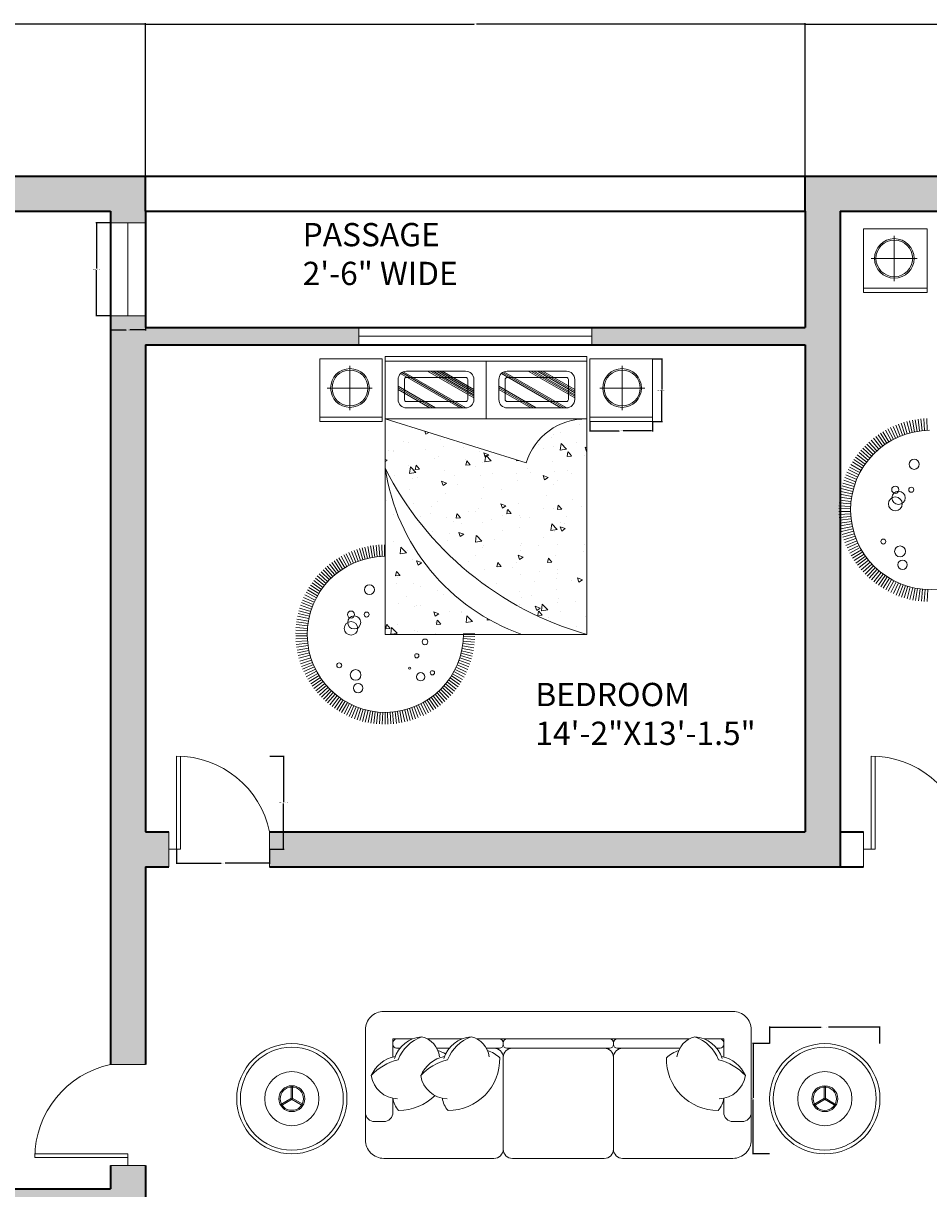
# Model space of a CAD drawing. Units: inches. Extents: x -9 to 646, y -802 to 47.
# Tile 16 of 17: x 191 to 424, y -253 to 47. Entities that reach past the tile are written whole.
import ezdxf

# ---------------------------------------------------------------- set-up
doc = ezdxf.new("R2010")
doc.units = ezdxf.units.IN
doc.header["$MEASUREMENT"] = 0
for name, color, linetype, lineweight in [('A-ANNO-DIMS', 2, 'Continuous', 18), ('A-AREA-IDEN', 7, 'Continuous', 18), ('A-DOOR', 4, 'Continuous', 18), ('A-FURN', 8, 'Continuous', 15), ('A-FURN-PATT', 252, 'Continuous', 9), ('A-GLAZ', 4, 'Continuous', 15), ('A-WALL', 7, 'Continuous', 35), ('A-WALL-PATT', 5, 'Continuous', 9)]:
    doc.layers.add(name, color=color, linetype=linetype, lineweight=lineweight)
doc.styles.get("Standard").update_dxf_attribs({"font": 'arial.ttf'})
doc.dimstyles.get("Standard").update_dxf_attribs({"dimtxt": 0.18, "dimasz": 0.18, "dimexe": 0.18, "dimexo": 0.0625, "dimgap": 0.09, "dimtad": 0, "dimtih": 1, "dimtoh": 1, "dimdec": 0, "dimzin": 0, "dimdsep": 46, "dimlunit": 3, "dimtxsty": 'Standard', "dimcen": 0.09, "dimadec": 0, "dimazin": 0, "dimtfac": 1, "dimtdec": 0, "dimtofl": 0, "dimtmove": 0, "dimatfit": 3, "dimfxl": 1, "dimtolj": 1, "dimtzin": 0, "dimarcsym": 0})

# ---------------------------------------------------------------- blocks, each defined once
blk = doc.blocks.new('END-TABLE-ROUND')
at = {"ltscale": 0.03}
for p, q in [((14.05, 14.2), (14.05, 17.54)), ((14.35, 14.2), (14.35, 17.54)), ((14.13, 14.33), (11.24, 12.66)), ((14.28, 14.07), (11.39, 12.4)), ((14.13, 14.07), (17.02, 12.4)), ((14.28, 14.33), (17.17, 12.66))]:
    blk.add_line(p, q, dxfattribs=at)
for radius in [14.21, 6.98, 3.34, 3]:
    blk.add_circle((14.2, 14.2), radius, dxfattribs=at)
blk.add_circle((14.2, 14.2), 13.26)
blk = doc.blocks.new('NIGHTSTAND-16')
for p, q in [((0, 0), (0, 16.11)), ((16.11, 16.11), (0, 16.11)), ((16.11, 16.11), (16.11, 0)), ((8.32, 14.34), (8.32, 2.9)), ((14.18, 8.62), (2.59, 8.62)), ((16.11, 1.13), (0, 1.13)), ((16.11, 0), (0, 0))]:
    blk.add_line(p, q)
for radius in [4.99, 4.63]:
    blk.add_circle((8.32, 8.62), radius)
blk = doc.blocks.new('NIGHTSTAND-16_5')
for p, q in [((0, 0), (0, 16.45)), ((16.45, 16.45), (0, 16.45)), ((16.45, 16.45), (16.45, 0)), ((8.49, 14.64), (8.49, 2.96)), ((14.48, 8.8), (2.64, 8.8)), ((16.45, 1.15), (0, 1.15)), ((16.45, 0), (0, 0))]:
    blk.add_line(p, q)
for radius in [5.09, 4.73]:
    blk.add_circle((8.49, 8.8), radius)
blk = doc.blocks.new('DOOR-LEAF-24-WALL9')
for p, q in [((0, 0), (0, 24)), ((1, 0), (1, 24)), ((0, 0), (1, 0))]:
    blk.add_line(p, q)
blk.add_arc((0, -0.52), 24.52, 11.8123, 90)
blk = doc.blocks.new('GLAZING-24')
for p, q in [((0, 9), (24, 9)), ((0, 4.5), (24, 4.5)), ((24, 0), (0, 0))]:
    blk.add_line(p, q)
blk = doc.blocks.new('*D21')
at = {"layer": 'A-ANNO-DIMS', "color": 0, "lineweight": -2, "transparency": 16777216}
for p, q in [((254.44, -141.57), (258.15, -141.57)), ((257.97, -141.75), (257.97, -153.39)), ((257.97, -165.39), (257.97, -153.75)), ((254.44, -165.57), (258.15, -165.57))]:
    blk.add_line(p, q, dxfattribs=at)
at = {"layer": 'A-ANNO-DIMS', "color": 0, "transparency": 16777216}
for points in [[(257.94, -141.75), (258, -141.75), (257.97, -141.57)], [(257.94, -165.39), (258, -165.39), (257.97, -165.57)]]:
    blk.add_solid(points, dxfattribs=at)
at = {"layer": 'Defpoints', "color": 0, "transparency": 16777216}
for p in [(254.37, -141.57), (257.97, -141.57), (254.37, -165.57)]:
    blk.add_point(p, dxfattribs=at)
at = {"layer": 'A-ANNO-DIMS', "color": 0, "transparency": 16777216, "insert": (257.97, -153.57), "char_height": 0.18, "attachment_point": 5}
blk.add_mtext('\\A1;DOOR LEAF 24 TYP.', dxfattribs=at)
blk = doc.blocks.new('*D22')
at = {"layer": 'A-ANNO-DIMS', "color": 0, "lineweight": -2, "transparency": 16777216}
for p, q in [((230.37, -165.63), (230.37, -169.35)), ((254.37, -165.63), (254.37, -169.35)), ((230.55, -169.17), (241.84, -169.17)), ((254.19, -169.17), (242.9, -169.17))]:
    blk.add_line(p, q, dxfattribs=at)
at = {"layer": 'A-ANNO-DIMS', "color": 0, "transparency": 16777216}
for points in [[(230.55, -169.14), (230.55, -169.2), (230.37, -169.17)], [(254.19, -169.14), (254.19, -169.2), (254.37, -169.17)]]:
    blk.add_solid(points, dxfattribs=at)
at = {"layer": 'Defpoints', "color": 0, "transparency": 16777216}
for p in [(230.37, -165.57), (254.37, -165.57), (254.37, -169.17)]:
    blk.add_point(p, dxfattribs=at)
at = {"layer": 'A-ANNO-DIMS', "color": 0, "transparency": 16777216, "insert": (242.37, -169.17), "char_height": 0.18, "attachment_point": 5}
blk.add_mtext('\\A1;24 TYP.', dxfattribs=at)
blk = doc.blocks.new('*D29')
at = {"layer": 'A-ANNO-DIMS', "color": 0, "lineweight": -2, "transparency": 16777216}
for p, q in [((213.31, -4.07), (209.59, -4.07)), ((209.77, -4.25), (209.77, -15.89)), ((209.77, -27.89), (209.77, -16.25)), ((213.31, -28.07), (209.59, -28.07))]:
    blk.add_line(p, q, dxfattribs=at)
at = {"layer": 'A-ANNO-DIMS', "color": 0, "transparency": 16777216}
for points in [[(209.74, -4.25), (209.8, -4.25), (209.77, -4.07)], [(209.74, -27.89), (209.8, -27.89), (209.77, -28.07)]]:
    blk.add_solid(points, dxfattribs=at)
at = {"layer": 'Defpoints', "color": 0, "transparency": 16777216}
for p in [(213.37, -4.07), (209.77, -28.07), (213.37, -28.07)]:
    blk.add_point(p, dxfattribs=at)
at = {"layer": 'A-ANNO-DIMS', "color": 0, "transparency": 16777216, "insert": (209.77, -16.07), "char_height": 0.18, "attachment_point": 5}
blk.add_mtext('\\A1;WINDOW 24 TYP.', dxfattribs=at)
blk = doc.blocks.new('*D30')
at = {"layer": 'A-ANNO-DIMS', "color": 0, "lineweight": -2, "transparency": 16777216}
for p, q in [((213.37, -28.13), (213.37, -31.85)), ((222.37, -28.13), (222.37, -31.85)), ((213.55, -31.67), (217.41, -31.67)), ((222.19, -31.67), (218.33, -31.67))]:
    blk.add_line(p, q, dxfattribs=at)
at = {"layer": 'A-ANNO-DIMS', "color": 0, "transparency": 16777216}
for points in [[(213.55, -31.64), (213.55, -31.7), (213.37, -31.67)], [(222.19, -31.64), (222.19, -31.7), (222.37, -31.67)]]:
    blk.add_solid(points, dxfattribs=at)
at = {"layer": 'Defpoints', "color": 0, "transparency": 16777216}
for p in [(213.37, -28.07), (222.37, -28.07), (222.37, -31.67)]:
    blk.add_point(p, dxfattribs=at)
at = {"layer": 'A-ANNO-DIMS', "color": 0, "transparency": 16777216, "insert": (217.87, -31.67), "char_height": 0.18, "attachment_point": 5}
blk.add_mtext('\\A1;9 TYP.', dxfattribs=at)
blk = doc.blocks.new('*D37')
at = {"layer": 'A-ANNO-DIMS', "color": 0, "lineweight": -2, "transparency": 16777216}
for p, q in [((383.2, -215.6), (383.2, -211.22)), ((383.38, -211.4), (396.44, -211.4)), ((411.43, -211.4), (398.37, -211.4)), ((411.61, -215.6), (411.61, -211.22))]:
    blk.add_line(p, q, dxfattribs=at)
at = {"layer": 'A-ANNO-DIMS', "color": 0, "transparency": 16777216}
for points in [[(383.38, -211.37), (383.38, -211.43), (383.2, -211.4)], [(411.43, -211.37), (411.43, -211.43), (411.61, -211.4)]]:
    blk.add_solid(points, dxfattribs=at)
at = {"layer": 'Defpoints', "color": 0, "transparency": 16777216}
for p in [(411.61, -211.4), (383.2, -215.66), (411.61, -215.66)]:
    blk.add_point(p, dxfattribs=at)
at = {"layer": 'A-ANNO-DIMS', "color": 0, "transparency": 16777216, "insert": (397.4, -211.4), "char_height": 0.18, "attachment_point": 5}
blk.add_mtext('\\A1;TABLE 28 TYP.', dxfattribs=at)
blk = doc.blocks.new('*D38')
at = {"layer": 'A-ANNO-DIMS', "color": 0, "lineweight": -2, "transparency": 16777216}
for p, q in [((383.14, -215.66), (378.76, -215.66)), ((378.94, -215.84), (378.94, -229.69)), ((378.94, -243.89), (378.94, -230.05)), ((383.14, -244.07), (378.76, -244.07))]:
    blk.add_line(p, q, dxfattribs=at)
at = {"layer": 'A-ANNO-DIMS', "color": 0, "transparency": 16777216}
for points in [[(378.91, -215.84), (378.97, -215.84), (378.94, -215.66)], [(378.91, -243.89), (378.97, -243.89), (378.94, -244.07)]]:
    blk.add_solid(points, dxfattribs=at)
at = {"layer": 'Defpoints', "color": 0, "transparency": 16777216}
for p in [(378.94, -215.66), (383.2, -215.66), (383.2, -244.07)]:
    blk.add_point(p, dxfattribs=at)
at = {"layer": 'A-ANNO-DIMS', "color": 0, "transparency": 16777216, "insert": (378.94, -229.87), "char_height": 0.18, "attachment_point": 5}
blk.add_mtext('\\A1;28 TYP.', dxfattribs=at)
blk = doc.blocks.new('*D43')
at = {"layer": 'A-ANNO-DIMS', "color": 0, "lineweight": -2, "transparency": 16777216}
for p, q in [((353.04, -39.17), (355.57, -39.17)), ((355.39, -39.35), (355.39, -47.04)), ((355.39, -55.1), (355.39, -47.41)), ((353.04, -55.28), (355.57, -55.28))]:
    blk.add_line(p, q, dxfattribs=at)
at = {"layer": 'A-ANNO-DIMS', "color": 0, "transparency": 16777216}
for points in [[(355.36, -39.35), (355.42, -39.35), (355.39, -39.17)], [(355.36, -55.1), (355.42, -55.1), (355.39, -55.28)]]:
    blk.add_solid(points, dxfattribs=at)
at = {"layer": 'Defpoints', "color": 0, "transparency": 16777216}
for p in [(352.97, -39.17), (355.39, -39.17), (352.97, -55.28)]:
    blk.add_point(p, dxfattribs=at)
at = {"layer": 'A-ANNO-DIMS', "color": 0, "transparency": 16777216, "insert": (355.39, -47.22), "char_height": 0.18, "attachment_point": 5}
blk.add_mtext('\\A1;NIGHTSTAND 16 TYP.', dxfattribs=at)
blk = doc.blocks.new('*D44')
at = {"layer": 'A-ANNO-DIMS', "color": 0, "lineweight": -2, "transparency": 16777216}
for p, q in [((336.86, -55.34), (336.86, -57.88)), ((352.97, -55.34), (352.97, -57.88)), ((337.04, -57.7), (344.4, -57.7)), ((352.79, -57.7), (345.44, -57.7))]:
    blk.add_line(p, q, dxfattribs=at)
at = {"layer": 'A-ANNO-DIMS', "color": 0, "transparency": 16777216}
for points in [[(337.04, -57.67), (337.04, -57.73), (336.86, -57.7)], [(352.79, -57.67), (352.79, -57.73), (352.97, -57.7)]]:
    blk.add_solid(points, dxfattribs=at)
at = {"layer": 'Defpoints', "color": 0, "transparency": 16777216}
for p in [(336.86, -55.28), (352.97, -55.28), (352.97, -57.7)]:
    blk.add_point(p, dxfattribs=at)
at = {"layer": 'A-ANNO-DIMS', "color": 0, "transparency": 16777216, "insert": (344.92, -57.7), "char_height": 0.18, "attachment_point": 5}
blk.add_mtext('\\A1;16 TYP.', dxfattribs=at)
blk = doc.blocks.new('*D51')
at = {"layer": 'A-ANNO-DIMS', "color": 0, "lineweight": -2, "transparency": 16777216}
for p, q in [((30.37, 7.99), (30.37, 47.36)), ((30.55, 47.18), (126.09, 47.18)), ((222.19, 47.18), (126.65, 47.18)), ((222.37, 7.99), (222.37, 47.36))]:
    blk.add_line(p, q, dxfattribs=at)
at = {"layer": 'A-ANNO-DIMS', "color": 0, "transparency": 16777216}
for points in [[(30.55, 47.21), (30.55, 47.15), (30.37, 47.18)], [(222.19, 47.21), (222.19, 47.15), (222.37, 47.18)]]:
    blk.add_solid(points, dxfattribs=at)
at = {"layer": 'Defpoints', "color": 0, "transparency": 16777216}
for p in [(222.37, 47.18), (30.37, 7.93), (222.37, 7.93)]:
    blk.add_point(p, dxfattribs=at)
at = {"layer": 'A-ANNO-DIMS', "color": 0, "transparency": 16777216, "insert": (126.37, 47.18), "char_height": 0.18, "attachment_point": 5}
blk.add_mtext('\\A1;192', dxfattribs=at)
blk = doc.blocks.new('*D52')
at = {"layer": 'A-ANNO-DIMS', "color": 0, "lineweight": -2, "transparency": 16777216}
for p, q in [((222.37, 7.99), (222.37, 47.36)), ((222.55, 47.18), (307.09, 47.18)), ((392.19, 47.18), (307.65, 47.18)), ((392.37, 7.99), (392.37, 47.36))]:
    blk.add_line(p, q, dxfattribs=at)
at = {"layer": 'A-ANNO-DIMS', "color": 0, "transparency": 16777216}
for points in [[(222.55, 47.21), (222.55, 47.15), (222.37, 47.18)], [(392.19, 47.21), (392.19, 47.15), (392.37, 47.18)]]:
    blk.add_solid(points, dxfattribs=at)
at = {"layer": 'Defpoints', "color": 0, "transparency": 16777216}
for p in [(392.37, 47.18), (222.37, 7.93), (392.37, 7.93)]:
    blk.add_point(p, dxfattribs=at)
at = {"layer": 'A-ANNO-DIMS', "color": 0, "transparency": 16777216, "insert": (307.37, 47.18), "char_height": 0.18, "attachment_point": 5}
blk.add_mtext('\\A1;170', dxfattribs=at)
blk = doc.blocks.new('*D53')
at = {"layer": 'A-ANNO-DIMS', "color": 0, "lineweight": -2, "transparency": 16777216}
for p, q in [((392.37, 7.99), (392.37, 47.36)), ((392.55, 47.18), (499.08, 47.18)), ((606.19, 47.18), (499.66, 47.18)), ((606.37, 7.99), (606.37, 47.36))]:
    blk.add_line(p, q, dxfattribs=at)
at = {"layer": 'A-ANNO-DIMS', "color": 0, "transparency": 16777216}
for points in [[(392.55, 47.21), (392.55, 47.15), (392.37, 47.18)], [(606.19, 47.21), (606.19, 47.15), (606.37, 47.18)]]:
    blk.add_solid(points, dxfattribs=at)
at = {"layer": 'Defpoints', "color": 0, "transparency": 16777216}
for p in [(606.37, 47.18), (392.37, 7.93), (606.37, 7.93)]:
    blk.add_point(p, dxfattribs=at)
at = {"layer": 'A-ANNO-DIMS', "color": 0, "transparency": 16777216, "insert": (499.37, 47.18), "char_height": 0.18, "attachment_point": 5}
blk.add_mtext('\\A1;214', dxfattribs=at)

msp = doc.modelspace()

# ---------------------------------------------------------------- hatches: boundary and pattern name
at = {"layer": 'A-FURN-PATT'}
h = msp.add_hatch(dxfattribs=at)
h.set_pattern_fill('ANSI31', color=256, scale=2.863983, angle=105.0416, style=0)
h.paths.add_polyline_path([(288.89, -42.45), (288.86, -42.46), (288.79, -42.48), (288.73, -42.51), (288.66, -42.54), (288.6, -42.57), (288.54, -42.61), (288.48, -42.64), (288.42, -42.68), (288.36, -42.72), (288.31, -42.76), (288.25, -42.81), (288.2, -42.85), (288.15, -42.9), (288.09, -42.95), (288.05, -42.99), (303.28, -51.77), (304.86, -51.77), (305.01, -51.76), (305.04, -51.76)])
h = msp.add_hatch(dxfattribs=at)
h.set_pattern_fill('ANSI31', color=256, scale=2.865408, angle=105.0416, style=0)
h.paths.add_polyline_path([(296.66, -42.32), (294.88, -42.32), (307.01, -49.31), (307.01, -48.28)])
h = msp.add_hatch(dxfattribs=at)
h.set_pattern_fill('ANSI31', color=256, scale=2.867606, angle=105.0416, style=0)
h.paths.add_polyline_path([(298.98, -42.32), (297.21, -42.32), (307.01, -47.97), (307.01, -46.94)])
h = msp.add_hatch(dxfattribs=at)
h.set_pattern_fill('ANSI31', color=256, scale=2.865794, angle=105.0416, style=0)
h.paths.add_polyline_path([(314.85, -42.45), (314.74, -42.49), (314.61, -42.55), (314.49, -42.61), (314.37, -42.69), (314.26, -42.77), (314.15, -42.85), (314.05, -42.95), (314.01, -42.99), (329.24, -51.77), (330.82, -51.77), (330.97, -51.76), (331, -51.76)])
h = msp.add_hatch(dxfattribs=at)
h.set_pattern_fill('ANSI31', color=256, scale=2.867013, angle=105.0416, style=0)
h.paths.add_polyline_path([(322.62, -42.32), (320.84, -42.32), (332.97, -49.31), (332.97, -48.28)])
h = msp.add_hatch(dxfattribs=at)
h.set_pattern_fill('ANSI31', color=256, scale=2.860774, angle=105.0416, style=0)
h.paths.add_polyline_path([(324.94, -42.32), (323.17, -42.32), (332.97, -47.97), (332.97, -46.94)])
h = msp.add_hatch(dxfattribs=at)
h.set_pattern_fill('ANSI31', color=256, scale=2.865341, angle=105.0416, style=0)
h.paths.add_polyline_path([(287.47, -46.12), (287.47, -47.14), (295.49, -51.77), (297.27, -51.77)])
h = msp.add_hatch(dxfattribs=at)
h.set_pattern_fill('ANSI31', color=256, scale=2.867063, angle=105.0416, style=0)
h.paths.add_polyline_path([(313.43, -46.12), (313.43, -47.14), (321.45, -51.77), (323.23, -51.77)])
h = msp.add_hatch(dxfattribs=at)
h.set_pattern_fill('AR-CONC', color=256, scale=0.071614, angle=180, style=0)
h.set_pattern_definition([(130, (947.846, -4102.651), (-13.047038, -1.141467), [1.364254, -15.00679]), (185, (947.846, -4102.651), (2.523892, 13.6824), [1.091403, -12.00543]), (79.549, (946.759, -4102.746), (-10.523193, 12.54087), [1.159436, -12.7538]), (133.8158, (947.846, -4099.013), (-19.41315, -3.010834), [2.04638, -22.51018]), (83.3644, (946.229, -4099.264), (-17.00155, 17.71922), [1.73915, -19.1307]), (188.816, (947.846, -4099.013), (-17.00158, 17.71919), [1.6371, -18.00815]), (159, (946.027, -4099.922), (-10.857802, -7.32368), [1.364254, -15.00679]), (214, (946.027, -4099.922), (-4.425913, 13.190503), [1.091403, -12.00543]), (108.5486, (945.123, -4100.532), (-15.283685, 5.866853), [1.159436, -12.7538]), (142.5, (947.8463, -4102.6507), (-0.2211883, 6.055355), [0, -11.85991, 0, -12.187331, 0, -12.050906]), (172.5, (947.846, -4102.651), (-4.785247, 7.174367), [0, -6.948598, 0, -11.58706, 0, -4.592987]), (212.5, (951.9027, -4102.6507), (-9.7102333, -0.4102603), [0, -4.547512, 0, -14.188236, 0, -18.826698]), (222.5, (953.722, -4102.651), (-10.608176, 1.820902), [0, -5.911765, 0, -9.422444, 0, -13.369684])])
edge = h.paths.add_edge_path()
edge.add_ellipse((335.77, -70.63), major_axis=(-11.32, 11.32), ratio=1, start_angle=-43.8468, end_angle=28.0453, ccw=False)
edge.add_line((335.44, -54.62), (336.09, -54.62))
edge.add_line((336.09, -54.62), (336.09, -110.16))
edge.add_ellipse((358.89, -29.61), major_axis=(-59.2, 59.2), ratio=1, start_angle=71.7955, end_angle=119.1914, ccw=False)
edge.add_line((284.17, -67.35), (284.17, -54.62))
edge.add_line((284.17, -54.62), (320.45, -65.96))
edge = h.paths.add_edge_path()
edge.add_line((319.34, -110.16), (284.17, -110.16))
edge.add_line((284.17, -110.16), (284.17, -67.35))
edge.add_ellipse((337.17, -59.66), major_axis=(37.87, 37.87), ratio=1, start_angle=143.2583, end_angle=205.5572)
at = {"layer": 'A-WALL-PATT'}
h = msp.add_hatch(color=256, dxfattribs=at)
h.dxf.hatch_style = 1
h.paths.add_polyline_path([(73.4, -418.07), (63.37, -418.07), (63.37, -487.07), (63.35, -496.07), (67.87, -496.07), (67.87, -427.07), (73.4, -427.07)])
h.paths.add_polyline_path([(73.87, -487.07), (67.87, -487.07), (67.87, -496.07), (73.87, -496.07)])
h.paths.add_polyline_path([(39.37, -496.07), (39.35, -496.07), (39.35, -487.07), (30.37, -487.07), (30.37, -646.07), (69.62, -646.07), (69.62, -637.07), (39.37, -637.07)])
h.paths.add_polyline_path([(158.27, -637.07), (105.62, -637.07), (105.62, -646.07), (158.27, -646.07)])
h.paths.add_polyline_path([(286.47, -637.07), (194.27, -637.07), (194.27, -646.07), (286.47, -646.07)])
h.paths.add_polyline_path([(357.37, -552.07), (352.87, -552.07), (348.37, -552.07), (348.37, -637.07), (322.47, -637.07), (322.47, -646.07), (357.37, -646.07)])
h.paths.add_polyline_path([(357.37, -459.07), (352.87, -459.07), (348.37, -459.07), (348.37, -526.07), (357.37, -526.07), (357.37, -520.07), (363.37, -520.07), (363.37, -511.07), (357.37, -511.07)], flags=17)
h.paths.add_polyline_path([(39.37, -262.07), (213.37, -262.07), (213.37, -268.07), (222.37, -268.07), (222.37, -247.07), (213.37, -247.07), (213.37, -253.07), (39.37, -253.07), (39.37, -1.07), (222.37, -1.07), (222.37, 7.93), (30.37, 7.93), (30.37, -427.07), (39.36, -427.07), (39.36, -418.07)])
h.paths.add_polyline_path([(570.37, -149.32), (561.37, -149.32), (561.37, -161.07), (433.37, -161.07), (433.37, -165.57), (433.37, -170.07), (438.37, -170.07), (438.37, -176.07), (447.37, -176.07), (447.37, -170.07), (561.37, -170.07), (561.37, -229.57), (570.37, -229.57)])
h.paths.add_polyline_path([(570.37, -289.57), (561.37, -289.57), (561.37, -349.07), (479.37, -349.07), (479.37, -353.57), (479.37, -358.07), (561.37, -358.07), (561.37, -418.07), (447.37, -418.07), (447.37, -358.07), (453.37, -358.07), (453.37, -349.07), (447.37, -349.07), (447.37, -202.07), (442.87, -202.07), (438.37, -202.07), (438.37, -427.07), (561.37, -427.07), (561.37, -451.07), (570.37, -451.07)])
h.paths.add_polyline_path([(570.37, -496.07), (570.37, -487.07), (561.37, -487.07), (561.37, -511.07), (411.37, -511.07), (411.37, -515.57), (411.37, -520.07), (570.37, -520.07)])
h = msp.add_hatch(color=256, dxfattribs=at)
h.dxf.hatch_style = 1
h.paths.add_polyline_path([(401.37, -1.07), (538.87, -1.07), (538.87, -7.07), (543.37, -7.07), (543.37, -1.07), (597.37, -1.07), (597.37, -97.07), (595.89, -97.07), (595.89, -101.57), (606.37, -101.57), (606.37, 7.93), (570.37, 7.93), (392.37, 7.93), (392.37, -1.07), (392.37, -31.07), (337.37, -31.07), (337.37, -35.57), (392.37, -35.57), (392.37, -161.07), (254.37, -161.07), (254.37, -165.57), (254.37, -170.07), (401.37, -170.07)])
h.paths.add_polyline_path([(228.37, -161.07), (222.37, -161.07), (222.37, -35.57), (277.37, -35.57), (277.37, -31.07), (222.37, -31.07), (222.37, -28.07), (213.37, -28.07), (213.37, -221.07), (217.87, -221.07), (222.37, -221.07), (222.37, -170.07), (228.37, -170.07)])
h.paths.add_polyline_path([(571.89, -97.07), (543.37, -97.07), (543.37, -33.07), (541.12, -33.07), (538.87, -33.07), (538.87, -101.57), (561.37, -101.57), (561.37, -113.32), (570.37, -113.32), (570.37, -101.57), (571.89, -101.57)], flags=17)
h = msp.add_hatch(color=256, dxfattribs=at)
h.dxf.hatch_style = 1
h.paths.add_polyline_path([(222.37, -1.07), (213.37, -1.07), (213.37, -4.07), (222.37, -4.07)])
h.paths.add_polyline_path([(222.37, -28.07), (213.37, -28.07), (213.37, -31.07), (222.37, -31.07)])

# ---------------------------------------------------------------- linework, layer by layer
at = {"layer": 'A-DOOR'}
for p, q in [((228.37, -161.07), (228.37, -170.07)), ((254.37, -165.57), (254.37, -161.07)), ((407.37, -161.07), (407.37, -170.07)), ((228.37, -165.57), (230.37, -165.57)), ((254.37, -165.57), (254.37, -170.07)), ((407.37, -165.57), (409.37, -165.57)), ((217.87, -221.07), (213.37, -221.07)), ((217.87, -221.07), (222.37, -221.07)), ((217.87, -247.07), (217.87, -245.07)), ((213.37, -247.07), (222.37, -247.07))]:
    msp.add_line(p, q, dxfattribs=at)
at = {"layer": 'A-FURN'}
for p, q in [((284.17, -110.16), (284.17, -38.55)), ((336.09, -38.55), (284.17, -38.55)), ((336.09, -38.55), (336.09, -110.16)), ((284.17, -39.72), (336.09, -39.72)), ((310.13, -54.62), (310.13, -39.72)), ((284.17, -54.62), (336.09, -54.62)), ((284.17, -54.62), (320.45, -65.96)), ((415.64, -59.61), (414.33, -56.85)), ((416.23, -59.34), (415, -56.54)), ((416.82, -59.08), (415.69, -56.25)), ((417.43, -58.85), (416.39, -55.97)), ((418.04, -58.63), (417.09, -55.73)), ((418.66, -58.43), (417.8, -55.5)), ((419.28, -58.25), (418.52, -55.3)), ((419.91, -58.09), (419.24, -55.12)), ((420.55, -57.96), (419.97, -54.96)), ((421.18, -57.84), (420.7, -54.82)), ((421.83, -57.74), (421.44, -54.71)), ((422.47, -57.66), (422.18, -54.62)), ((423.12, -57.61), (422.92, -54.56)), ((423.77, -57.57), (423.67, -54.52)), ((411.8, -62.03), (409.92, -59.62)), ((412.31, -61.63), (410.51, -59.17)), ((412.84, -61.25), (411.11, -58.73)), ((413.38, -60.89), (411.73, -58.32)), ((413.93, -60.54), (412.36, -57.92)), ((414.49, -60.21), (413.01, -57.54)), ((415.06, -59.9), (413.66, -57.19)), ((409, -64.73), (406.7, -62.72)), ((409.43, -64.24), (407.19, -62.17)), ((409.88, -63.77), (407.7, -61.62)), ((410.34, -63.31), (408.23, -61.1)), ((410.81, -62.87), (408.78, -60.59)), ((411.3, -62.44), (409.34, -60.1)), ((407.09, -67.35), (404.5, -65.73)), ((407.44, -66.8), (404.9, -65.1)), ((407.81, -66.27), (405.32, -64.49)), ((408.19, -65.74), (405.76, -63.89)), ((408.59, -65.23), (406.22, -63.3)), ((405.62, -70.24), (402.81, -69.05)), ((405.88, -69.65), (403.1, -68.37)), ((406.15, -69.06), (403.42, -67.69)), ((406.45, -68.48), (403.76, -67.03)), ((406.76, -67.91), (404.12, -66.37)), ((404.78, -72.7), (401.84, -71.87)), ((404.96, -72.07), (402.05, -71.16)), ((405.16, -71.46), (402.28, -70.45)), ((405.38, -70.85), (402.53, -69.74)), ((404.26, -75.24), (401.24, -74.79)), ((404.36, -74.6), (401.36, -74.05)), ((404.48, -73.96), (401.5, -73.32)), ((404.62, -73.33), (401.66, -72.59)), ((404.07, -77.83), (401.01, -77.76)), ((404.08, -77.18), (401.03, -77.02)), ((404.12, -76.53), (401.08, -76.27)), ((404.18, -75.89), (401.15, -75.53)), ((404.07, -78.48), (401.01, -78.51)), ((404.09, -79.13), (401.04, -79.26)), ((404.13, -79.77), (401.09, -80)), ((404.2, -80.42), (401.16, -80.74)), ((404.28, -81.06), (401.26, -81.48)), ((404.39, -81.71), (401.38, -82.22)), ((404.51, -82.34), (401.52, -82.95)), ((404.65, -82.98), (401.68, -83.68)), ((404.82, -83.6), (401.87, -84.4)), ((282.72, -90.11), (282.53, -87.12)), ((283.36, -90.07), (283.26, -87.08)), ((283.99, -90.06), (283.99, -87.06)), ((405, -84.23), (402.08, -85.11)), ((405.21, -84.84), (402.32, -85.82)), ((405.43, -85.45), (402.57, -86.52)), ((405.67, -86.05), (402.85, -87.22)), ((405.94, -86.65), (403.15, -87.9)), ((274.27, -92.66), (272.82, -90.04)), ((274.83, -92.36), (273.46, -89.7)), ((275.4, -92.07), (274.11, -89.37)), ((275.97, -91.8), (274.78, -89.06)), ((276.56, -91.55), (275.45, -88.77)), ((277.15, -91.32), (276.13, -88.51)), ((277.75, -91.11), (276.82, -88.26)), ((278.35, -90.91), (277.51, -88.04)), ((278.97, -90.74), (278.22, -87.84)), ((279.58, -90.58), (278.93, -87.67)), ((280.2, -90.45), (279.64, -87.51)), ((280.83, -90.33), (280.36, -87.38)), ((281.46, -90.24), (281.08, -87.27)), ((282.09, -90.16), (281.81, -87.19)), ((406.22, -87.23), (403.47, -88.57)), ((406.51, -87.81), (403.81, -89.23)), ((406.83, -88.38), (404.18, -89.89)), ((407.17, -88.93), (404.56, -90.53)), ((407.52, -89.48), (404.96, -91.15)), ((407.89, -90.01), (405.39, -91.77)), ((270.67, -95.26), (268.68, -93.03)), ((271.15, -94.84), (269.23, -92.55)), ((271.64, -94.44), (269.79, -92.08)), ((272.14, -94.05), (270.37, -91.64)), ((272.66, -93.68), (270.97, -91.21)), ((273.18, -93.32), (271.57, -90.8)), ((273.72, -92.98), (272.19, -90.41)), ((408.27, -90.54), (405.83, -92.37)), ((408.67, -91.05), (406.29, -92.95)), ((409.09, -91.54), (406.77, -93.53)), ((409.52, -92.03), (407.27, -94.08)), ((409.97, -92.5), (407.78, -94.62)), ((410.44, -92.95), (408.31, -95.14)), ((268.49, -97.57), (266.17, -95.68)), ((268.9, -97.08), (266.64, -95.12)), ((269.32, -96.61), (267.13, -94.57)), ((269.75, -96.14), (267.63, -94.04)), ((270.2, -95.69), (268.15, -93.52)), ((410.91, -93.39), (408.86, -95.65)), ((411.4, -93.82), (409.42, -96.14)), ((411.91, -94.23), (410, -96.61)), ((412.43, -94.62), (410.59, -97.06)), ((412.95, -95), (411.2, -97.5)), ((413.5, -95.35), (411.82, -97.91)), ((414.05, -95.7), (412.46, -98.3)), ((414.61, -96.02), (413.1, -98.68)), ((266.7, -100.2), (264.12, -98.69)), ((267.03, -99.65), (264.49, -98.06)), ((267.37, -99.11), (264.88, -97.45)), ((267.73, -98.59), (265.3, -96.85)), ((268.1, -98.07), (265.73, -96.26)), ((415.18, -96.33), (413.76, -99.03)), ((415.76, -96.62), (414.43, -99.36)), ((416.35, -96.89), (415.1, -99.67)), ((416.95, -97.14), (415.75, -100.07)), ((417.56, -97.37), (416.45, -100.33)), ((418.17, -97.58), (417.16, -100.57)), ((418.79, -97.78), (417.88, -100.79)), ((419.42, -97.95), (418.6, -100.99)), ((420.05, -98.1), (419.33, -101.16)), ((420.68, -98.24), (420.06, -101.31)), ((421.32, -98.35), (420.8, -101.44)), ((421.97, -98.44), (421.54, -101.54)), ((422.61, -98.52), (422.28, -101.62)), ((423.26, -98.57), (423.03, -101.68)), ((423.91, -98.6), (423.77, -101.71)), ((265.35, -103.07), (262.56, -101.99)), ((265.59, -102.48), (262.83, -101.31)), ((265.84, -101.9), (263.12, -100.64)), ((266.11, -101.32), (263.43, -99.98)), ((266.4, -100.75), (263.77, -99.33)), ((264.61, -105.5), (261.71, -104.78)), ((264.77, -104.89), (261.89, -104.08)), ((264.94, -104.28), (262.09, -103.38)), ((265.14, -103.67), (262.32, -102.68)), ((264.18, -108.01), (261.21, -107.66)), ((264.26, -107.38), (261.3, -106.94)), ((264.35, -106.75), (261.41, -106.21)), ((264.47, -106.12), (261.55, -105.5)), ((264.06, -109.91), (261.07, -109.85)), ((264.07, -110.55), (261.08, -110.58)), ((264.08, -109.27), (261.09, -109.12)), ((264.12, -108.64), (261.14, -108.39)), ((336.09, -110.16), (284.17, -110.16)), ((304.27, -109.99), (307.26, -109.99)), ((304.27, -110.62), (307.26, -110.72)), ((264.09, -111.18), (261.1, -111.31)), ((264.13, -111.82), (261.15, -112.04)), ((264.19, -112.45), (261.22, -112.76)), ((264.27, -113.08), (261.31, -113.49)), ((264.38, -113.71), (261.43, -114.21)), ((303.94, -113.78), (306.88, -114.34)), ((304.05, -113.15), (307, -113.62)), ((304.13, -112.52), (307.1, -112.9)), ((304.2, -111.89), (307.17, -112.17)), ((304.24, -111.26), (307.23, -111.45)), ((264.5, -114.33), (261.57, -114.93)), ((264.64, -114.95), (261.73, -115.64)), ((264.8, -115.57), (261.91, -116.34)), ((264.98, -116.18), (262.12, -117.05)), ((265.18, -116.78), (262.35, -117.74)), ((303.13, -116.85), (305.94, -117.87)), ((303.33, -116.25), (306.17, -117.18)), ((303.51, -115.64), (306.38, -116.48)), ((303.67, -115.02), (306.57, -115.77)), ((303.82, -114.4), (306.74, -115.06)), ((265.4, -117.38), (262.6, -118.43)), ((265.64, -117.97), (262.87, -119.1)), ((265.89, -118.55), (263.17, -119.77)), ((266.17, -119.12), (263.48, -120.43)), ((266.46, -119.69), (263.82, -121.08)), ((301.84, -119.75), (304.45, -121.2)), ((302.13, -119.19), (304.79, -120.55)), ((302.41, -118.62), (305.11, -119.9)), ((302.67, -118.03), (305.41, -119.23)), ((302.91, -117.45), (305.68, -118.55)), ((266.77, -120.24), (264.17, -121.72)), ((267.1, -120.79), (264.55, -122.34)), ((267.44, -121.32), (264.94, -122.96)), ((267.81, -121.84), (265.36, -123.56)), ((268.18, -122.36), (265.79, -124.15)), ((268.58, -122.85), (266.24, -124.72)), ((299.71, -122.91), (302.01, -124.83)), ((300.11, -122.41), (302.46, -124.26)), ((300.48, -121.9), (302.9, -123.67)), ((300.85, -121.38), (303.31, -123.07)), ((301.19, -120.85), (303.71, -122.46)), ((301.52, -120.31), (304.09, -121.84)), ((268.99, -123.34), (266.71, -125.28)), ((269.41, -123.81), (267.2, -125.83)), ((269.85, -124.27), (267.7, -126.36)), ((270.3, -124.72), (268.22, -126.87)), ((270.77, -125.15), (268.76, -127.36)), ((271.25, -125.57), (269.31, -127.84)), ((271.74, -125.97), (269.88, -128.3)), ((296.53, -126.01), (298.35, -128.39)), ((297.03, -125.62), (298.92, -127.93)), ((297.51, -125.2), (299.47, -127.46)), ((297.98, -124.77), (300.01, -126.96)), ((298.43, -124.33), (300.54, -126.45)), ((298.87, -123.87), (301.04, -125.93)), ((299.3, -123.4), (301.53, -125.39)), ((272.25, -126.35), (270.46, -128.75)), ((272.77, -126.72), (271.05, -129.17)), ((273.3, -127.07), (271.66, -129.58)), ((273.84, -127.41), (272.28, -129.96)), ((274.39, -127.73), (272.91, -130.33)), ((274.95, -128.03), (273.56, -130.67)), ((275.52, -128.31), (274.21, -131)), ((276.1, -128.57), (274.87, -131.3)), ((276.68, -128.82), (275.5, -131.69)), ((277.28, -129.05), (276.19, -131.95)), ((290.99, -129.07), (291.98, -131.91)), ((291.58, -128.85), (292.66, -131.64)), ((292.17, -128.6), (293.23, -131.12)), ((292.75, -128.34), (294, -131.06)), ((293.32, -128.06), (294.66, -130.74)), ((293.88, -127.76), (295.3, -130.39)), ((294.43, -127.45), (295.94, -130.03)), ((294.97, -127.11), (296.56, -129.65)), ((295.5, -126.76), (297.17, -129.25)), ((296.02, -126.4), (297.77, -128.83)), ((277.88, -129.26), (276.89, -132.18)), ((278.49, -129.45), (277.59, -132.4)), ((279.1, -129.62), (278.3, -132.59)), ((279.72, -129.77), (279.01, -132.76)), ((280.34, -129.9), (279.73, -132.9)), ((280.96, -130.01), (280.45, -133.03)), ((281.59, -130.1), (281.18, -133.13)), ((282.22, -130.17), (281.9, -133.21)), ((282.86, -130.22), (282.63, -133.26)), ((283.49, -130.25), (283.37, -133.3)), ((284.13, -130.27), (284.1, -133.31)), ((284.77, -130.26), (284.83, -133.29)), ((285.4, -130.23), (285.56, -133.26)), ((286.03, -130.18), (286.29, -133.2)), ((286.67, -130.11), (287.02, -133.11)), ((287.3, -130.02), (287.74, -133.01)), ((287.92, -129.91), (288.46, -132.88)), ((288.55, -129.78), (289.18, -132.73)), ((289.16, -129.63), (289.89, -132.56)), ((289.78, -129.47), (290.59, -132.36)), ((290.38, -129.28), (291.29, -132.14))]:
    msp.add_line(p, q, dxfattribs=at)
for points in [[(304.86, -42.32), (289.61, -42.32, 0.414214), (287.47, -44.47), (287.47, -49.62, 0.414214), (289.61, -51.77), (304.86, -51.77, 0.414214), (307.01, -49.62), (307.01, -44.47, 0.414214)], [(304.86, -43.93), (289.61, -43.93, 0.414214), (289.08, -44.47), (289.08, -49.62, 0.414214), (289.61, -50.16), (304.86, -50.16, 0.414214), (305.4, -49.62), (305.4, -44.47, 0.414214)], [(330.82, -42.32), (315.57, -42.32, 0.414214), (313.43, -44.47), (313.43, -49.62, 0.414214), (315.57, -51.77), (330.82, -51.77, 0.414214), (332.97, -49.62), (332.97, -44.47, 0.414214)], [(330.82, -43.93), (315.57, -43.93, 0.414214), (315.04, -44.47), (315.04, -49.62, 0.414214), (315.57, -50.16), (330.82, -50.16, 0.414214), (331.36, -49.62), (331.36, -44.47, 0.414214)], [(315.49, -214.48), (342, -214.48, -0.414214), (342.95, -215.43), (342.95, -215.9, -0.414214), (342, -216.85), (315.49, -216.85, -0.414214), (314.54, -215.9), (314.54, -215.43, -0.414214)]]:
    msp.add_lwpolyline(points, format="xyb", close=True, dxfattribs=at)
at = {"layer": 'A-FURN', "ltscale": 0.03}
msp.add_lwpolyline([(378.46, -240.52, -0.414214), (373.73, -245.26), (345.32, -245.26, -0.414214), (342.95, -242.89, -0.414214), (340.58, -245.26), (316.91, -245.26, -0.414214), (314.54, -242.89, -0.414214), (312.17, -245.26), (283.76, -245.26, -0.414214), (279.03, -240.52), (279.03, -212.11, -0.414214), (283.76, -207.38), (373.73, -207.38, -0.414214), (378.46, -212.11)], format="xyb", close=True, dxfattribs=at)
at = {"layer": 'A-FURN'}
for points in [[(280.53, -223.93, -0.14773), (287.45, -219.86, -0.213343), (293.56, -213.89, -0.178662)], [(291.11, -214.48), (286.13, -214.48), (286.13, -219.13, -0.414214)], [(287.94, -216.85), (287.08, -216.85, -0.414214), (286.13, -215.9), (286.13, -215.43, -0.414214), (287.08, -214.48)], [(286.5, -219.53, -0.306663), (293.56, -213.89, -0.30633), (298.17, -219.05, 0.872847)], [(287.08, -214.48), (291.11, -214.48, -0.414214)], [(293.29, -223.93, -0.14773), (300.21, -219.86, -0.213343), (306.31, -213.89, -0.178662)], [(295.05, -214.48), (303.87, -214.48, -0.414214)], [(299.25, -219.53, -0.306663), (306.31, -213.89, -0.30633), (310.93, -219.05, 0.872847)], [(307.8, -214.48), (313.59, -214.48, -0.414214), (314.54, -215.43), (314.54, -215.9, -0.414214), (313.59, -216.85), (310.19, -216.85, -0.414214)], [(362.44, -214.48), (343.9, -214.48, 0.414214), (342.95, -215.43), (342.95, -215.9, 0.414214), (343.9, -216.85), (360.06, -216.85, 0.414214)], [(370.99, -219.53, 0.306663), (363.93, -213.89, 0.30633), (359.32, -219.05, -0.872847)], [(376.96, -223.93, 0.14773), (370.04, -219.86, 0.213343), (363.93, -213.89, 0.178662)], [(370.41, -214.48), (366.38, -214.48, 0.414214)], [(369.55, -216.85), (370.41, -216.85, 0.414214), (371.36, -215.9), (371.36, -215.43, 0.414214), (370.41, -214.48)], [(287.32, -229.9, -0.356772), (280.53, -223.93, -0.249542), (286.68, -219.01, 9.61688)], [(300.07, -229.9, -0.356772), (293.29, -223.93, -0.249542), (299.44, -219.01, 9.61688)], [(300.69, -216.85), (297.43, -216.85, -0.414214)], [(299.72, -218.37, 0.071865), (297.73, -217.45, -7.115464)], [(298.88, -229.75, 0.165541), (300.34, -232.88, 0.425989), (313.64, -219.32, 0.121523), (310.48, -217.45, -7.115464)], [(312.17, -216.85, -0.414214), (314.54, -219.22), (314.54, -242.89, -0.414214)], [(316.91, -216.85, 0.414214), (314.54, -219.22)], [(340.58, -216.85, -0.414214), (342.95, -219.22)], [(345.32, -216.85, 0.414214), (342.95, -219.22), (342.95, -242.89, 0.414214)], [(371.37, -229.75, -0.165541), (369.9, -232.88, -0.425989), (356.61, -219.32, -0.121523), (359.76, -217.45, 7.115464)], [(370.17, -229.9, 0.356772), (376.96, -223.93, 0.249542), (370.81, -219.01, -9.61688)], [(286.13, -229.75), (286.13, -233.42, -0.414214), (283.76, -235.79), (281.4, -235.79, -0.414214), (279.03, -233.42)], [(286.13, -229.75, 0.165541), (287.59, -232.88, 0.200231), (296.99, -229.07, 0.121523)], [(378.46, -233.42, -0.414214), (376.1, -235.79), (373.73, -235.79, -0.414214), (371.36, -233.42), (371.36, -229.75)]]:
    msp.add_lwpolyline(points, format="xyb", dxfattribs=at)
for points in [[(303.87, -214.48), (295.05, -214.48)], [(362.44, -214.48), (307.8, -214.48)], [(371.36, -219.13), (371.36, -214.48), (366.38, -214.48)]]:
    msp.add_lwpolyline(points, dxfattribs=at)
for centre, radius in [((420.43, -66.33), 1.31), ((415.57, -72.88), 0.934), ((415.57, -76.53), 1.78), ((416.41, -74.96), 1.71), ((419.68, -72.88), 0.646), ((412.48, -86.24), 0.646), ((416.79, -88.77), 1.4), ((417.43, -92.24), 1.22), ((280.09, -98.65), 1.28), ((275.33, -105.06), 0.914), ((279.35, -105.06), 0.633), ((275.33, -108.63), 1.74), ((276.15, -107.1), 1.67), ((294.39, -112.12), 0.739), ((292.28, -115.69), 0.545), ((272.3, -118.15), 0.633), ((276.52, -120.63), 1.37), ((290.45, -118.89), 0.264), ((293.28, -121.09), 1.09), ((296.31, -120.08), 0.545), ((277.15, -124.02), 1.2)]:
    msp.add_circle(centre, radius, dxfattribs=at)
for centre, radius, start, end in [((335.77, -70.63), 16.01, 88.8468, 163.0453), ((424.59, -78.08), 20.53, 90.4973, 0.4973), ((358.89, -29.61), 83.72, 206.7955, 254.1914), ((337.17, -59.66), 53.56, 188.2583, 250.5572), ((284.17, -110.16), 20.11, 90.4973, 0.4973)]:
    msp.add_arc(centre, radius, start, end, dxfattribs=at)
at = {"layer": 'A-GLAZ'}
for p, q in [((222.37, -4.07), (213.37, -4.07)), ((213.37, -28.07), (222.37, -28.07)), ((337.37, -31.07), (277.37, -31.07)), ((277.37, -31.07), (277.37, -35.57)), ((337.37, -35.57), (337.37, -31.07)), ((277.37, -33.32), (337.37, -33.32)), ((277.37, -35.57), (337.37, -35.57))]:
    msp.add_line(p, q, dxfattribs=at)
at = {"layer": 'A-WALL'}
for p, q in [((30.37, 7.93), (570.37, 7.93)), ((222.37, -1.07), (222.37, 7.93)), ((392.37, -1.07), (392.37, 7.93)), ((39.37, -1.07), (213.37, -1.07)), ((213.37, -1.07), (213.37, -221.07)), ((222.37, -1.07), (222.37, -31.07)), ((222.37, -1.07), (392.37, -1.07)), ((392.37, -1.07), (392.37, -31.07)), ((401.37, -1.07), (401.37, -170.07)), ((401.37, -1.07), (538.87, -1.07)), ((222.37, -31.07), (392.37, -31.07)), ((222.37, -35.57), (392.37, -35.57)), ((222.37, -35.57), (222.37, -161.07)), ((392.37, -35.57), (392.37, -161.07)), ((222.37, -161.07), (228.37, -161.07)), ((254.37, -161.07), (392.37, -161.07)), ((401.37, -161.07), (407.37, -161.07)), ((222.37, -170.07), (228.37, -170.07)), ((222.37, -170.07), (222.37, -221.07)), ((254.37, -170.07), (407.37, -170.07)), ((213.37, -247.07), (213.37, -253.07)), ((222.37, -247.07), (222.37, -268.07)), ((39.37, -253.07), (213.37, -253.07))]:
    msp.add_line(p, q, dxfattribs=at)

# ---------------------------------------------------------------- block references
at = {"layer": 'A-DOOR'}
for p in [(230.37, -165.57), (409.37, -165.57)]:
    msp.add_blockref('DOOR-LEAF-24-WALL9', p, dxfattribs=at)
at = {"layer": 'A-DOOR', "rotation": 89.99999999999996}
msp.add_blockref('DOOR-LEAF-24-WALL9', (217.87, -245.07), dxfattribs=at)
at = {"layer": 'A-FURN', "extrusion": (0, 0, -1), "zscale": -1}
for name, p in [('NIGHTSTAND-16_5', (-423.8, -22.04)), ('NIGHTSTAND-16', (-283.39, -55.28))]:
    msp.add_blockref(name, p, dxfattribs=at)
at = {"layer": 'A-FURN'}
for name, p in [('NIGHTSTAND-16', (336.86, -55.28)), ('END-TABLE-ROUND', (383.2, -244.07))]:
    msp.add_blockref(name, p, dxfattribs=at)
at = {"layer": 'A-FURN', "rotation": 239.999999997015}
msp.add_blockref('END-TABLE-ROUND', (254.89, -210.47), dxfattribs=at)
at = {"layer": 'A-GLAZ', "rotation": 270.0000000000002}
msp.add_blockref('GLAZING-24', (213.37, -4.07), dxfattribs=at)

# ---------------------------------------------------------------- texts
at = {"layer": 'A-AREA-IDEN', "char_height": 6, "attachment_point": 1}
for s, insert in [('PASSAGE\\P2\'-6" WIDE', (262.87, -4.12)), ('BEDROOM\\P14\'-2"X13\'-1.5"', (322.83, -122.67))]:
    msp.add_mtext(s, dxfattribs=dict(at, insert=insert))

# ---------------------------------------------------------------- dimensions: what is measured, and where the dimension line sits
at = {"layer": 'A-ANNO-DIMS'}
for base, p1, p2, picture, middle in [((222.37, 47.18), (30.37, 7.93), (222.37, 7.93), '*D51', (126.37, 47.18)), ((392.37, 47.18), (222.37, 7.93), (392.37, 7.93), '*D52', (307.37, 47.18)), ((606.37, 47.18), (392.37, 7.93), (606.37, 7.93), '*D53', (499.37, 47.18))]:
    dim = msp.add_linear_dim(base=base, p1=p1, p2=p2, dimstyle='Standard', override={"dimdec": 0, "dimlfac": 1, "dimrnd": 0, "dimzin": 0, "dimdsep": 46, "dimlunit": 2}, dxfattribs=at)
    dim.commit()
    dim.dimension.update_dxf_attribs({"geometry": picture, "text_midpoint": middle})
for base, p1, p2, angle, text, picture, middle in [((209.77, -28.07), (213.37, -4.07), (213.37, -28.07), 270, 'WINDOW <> TYP.', '*D29', (209.77, -16.07)), ((222.37, -31.67), (213.37, -28.07), (222.37, -28.07), 0, '<> TYP.', '*D30', (217.87, -31.67)), ((355.39, -39.17), (352.97, -55.28), (352.97, -39.17), 90, 'NIGHTSTAND <> TYP.', '*D43', (355.39, -47.22)), ((257.97, -141.57), (254.37, -165.57), (254.37, -141.57), 90, 'DOOR LEAF <> TYP.', '*D21', (257.97, -153.57)), ((378.94, -215.66), (383.2, -244.07), (383.2, -215.66), 90, '<> TYP.', '*D38', (378.94, -229.87))]:
    dim = msp.add_linear_dim(base=base, p1=p1, p2=p2, angle=angle, text=text, dimstyle='Standard', override={"dimdec": 0, "dimlfac": 1, "dimrnd": 0, "dimzin": 0, "dimdsep": 46, "dimlunit": 2}, dxfattribs=at)
    dim.commit()
    dim.dimension.update_dxf_attribs({"geometry": picture, "text_midpoint": middle})
for base, p1, p2, text, picture, middle in [((352.97, -57.7), (336.86, -55.28), (352.97, -55.28), '<> TYP.', '*D44', (344.92, -57.7)), ((254.37, -169.17), (230.37, -165.57), (254.37, -165.57), '<> TYP.', '*D22', (242.37, -169.17)), ((411.61, -211.4), (383.2, -215.66), (411.61, -215.66), 'TABLE <> TYP.', '*D37', (397.4, -211.4))]:
    dim = msp.add_linear_dim(base=base, p1=p1, p2=p2, text=text, dimstyle='Standard', override={"dimdec": 0, "dimlfac": 1, "dimrnd": 0, "dimzin": 0, "dimdsep": 46, "dimlunit": 2}, dxfattribs=at)
    dim.commit()
    dim.dimension.update_dxf_attribs({"geometry": picture, "text_midpoint": middle})

doc.saveas('drawing.dxf')
